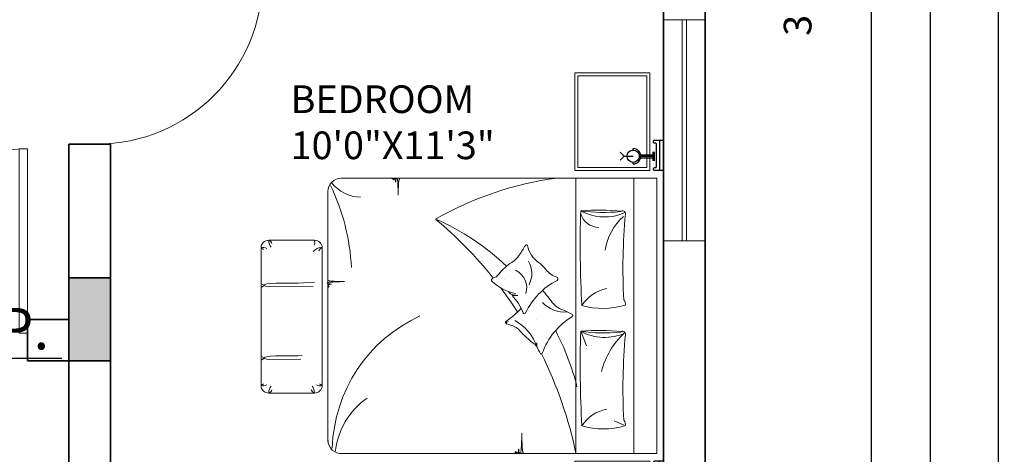
# Model space of a CAD drawing. Units: inches. Extents: x 3321 to 5237, y 11 to 1752.
# Tile 6 of 43: x 3652 to 3866, y 1204 to 1298. Entities that reach past the tile are written whole.
import ezdxf

# ---------------------------------------------------------------- set-up
doc = ezdxf.new("R2010")
doc.units = ezdxf.units.IN
for name, color, linetype, lineweight in [('A-ANNO-DIMS', 2, 'Continuous', 18), ('A-ANNO-TEXT', 7, 'Continuous', 18), ('A-AREA-IDEN', 7, 'Continuous', 18), ('A-COLS', 1, 'Continuous', 35), ('A-DOOR', 4, 'Continuous', 18), ('A-GLAZ', 5, 'Continuous', 18), ('A-WALL', 7, 'Continuous', 35), ('C-PROP', 7, 'Continuous', 30), ('FUR', 42, 'Continuous', 18)]:
    doc.layers.add(name, color=color, linetype=linetype, lineweight=lineweight)
for name, color, linetype in [('CEIL', 4, 'Continuous'), ('ELEC', 4, 'Continuous'), ('wood', 26, 'Continuous')]:
    doc.layers.add(name, color=color, linetype=linetype)
doc.styles.get("Standard").update_dxf_attribs({"font": 'arial.ttf'})
doc.dimstyles.new('ISO-25', dxfattribs={"dimtxt": 9, "dimasz": 2.5, "dimexe": 1.25, "dimexo": 0.625, "dimtad": 1, "dimdec": 1, "dimlunit": 3, "dimtxsty": 'Standard', "dimcen": 2.5, "dimclrd": 4, "dimclre": 4, "dimclrt": 256, "dimadec": 0, "dimazin": 0, "dimtfac": 1, "dimtdec": 1, "dimtmove": 0, "dimatfit": 3, "dimfxl": 1, "dimarcsym": 0})

# ---------------------------------------------------------------- blocks, each defined once
blk = doc.blocks.new('*U2')
for p, q in [((0, 0), (0, -6)), ((-40, 0), (-40, -6))]:
    blk.add_line(p, q)
blk.add_lwpolyline([(0, 0), (0, 40), (-1.75, 40), (-1.75, 0)], close=True)
blk.add_arc((0, 0), 40, 90, 180)
blk = doc.blocks.new('*U3')
for p, q in [((0, 0), (0, -6)), ((36, 0), (36, -6))]:
    blk.add_line(p, q)
blk.add_lwpolyline([(0, 0), (0, 36), (1.75, 36), (1.75, 0)], close=True)
blk.add_arc((0, 0), 36, 0, 90)
blk = doc.blocks.new('*D42')
at = {"layer": 'A-ANNO-DIMS', "color": 0, "lineweight": -2, "transparency": 16777216}
for p, q in [((3837.31, 1635.34), (3850.8, 1635.34)), ((3849.55, 1632.84), (3849.55, 1093.84)), ((3837.31, 1091.34), (3850.8, 1091.34))]:
    blk.add_line(p, q, dxfattribs=at)
at = {"layer": 'A-ANNO-DIMS', "color": 0, "transparency": 16777216}
for points in [[(3849.13, 1632.84), (3849.96, 1632.84), (3849.55, 1635.34)], [(3849.13, 1093.84), (3849.96, 1093.84), (3849.55, 1091.34)]]:
    blk.add_solid(points, dxfattribs=at)
at = {"layer": 'Defpoints', "color": 0, "transparency": 16777216}
for p in [(3836.69, 1635.34), (3836.69, 1091.34), (3849.55, 1091.34)]:
    blk.add_point(p, dxfattribs=at)
at = {"layer": 'A-ANNO-DIMS', "color": 0, "transparency": 16777216, "insert": (3844.35, 1363.34), "char_height": 9, "attachment_point": 5, "rotation": 90}
blk.add_mtext('45\'-4"', dxfattribs=at)
blk = doc.blocks.new('*D47')
at = {"layer": 'A-ANNO-DIMS', "color": 0, "lineweight": -2, "transparency": 16777216}
for p, q in [((3837.31, 1707.34), (3865.6, 1707.34)), ((3864.35, 989.84), (3864.35, 1704.84)), ((3837.31, 987.34), (3865.6, 987.34))]:
    blk.add_line(p, q, dxfattribs=at)
at = {"layer": 'A-ANNO-DIMS', "color": 0, "transparency": 16777216}
for points in [[(3863.93, 1704.84), (3864.76, 1704.84), (3864.35, 1707.34)], [(3863.93, 989.84), (3864.76, 989.84), (3864.35, 987.34)]]:
    blk.add_solid(points, dxfattribs=at)
at = {"layer": 'Defpoints', "color": 0, "transparency": 16777216}
for p in [(3836.69, 1707.34), (3864.35, 1707.34), (3836.69, 987.34)]:
    blk.add_point(p, dxfattribs=at)
at = {"layer": 'A-ANNO-DIMS', "color": 0, "transparency": 16777216, "insert": (3859.13, 1347.34), "char_height": 9, "attachment_point": 5, "rotation": 90}
blk.add_mtext("60'", dxfattribs=at)
blk = doc.blocks.new('*X127')
at = {"color": 0}
for p, q in [((3155.9, 8182.9), (3155.9, 8182.9)), ((3147.8, 8143.4), (3147.8, 8143.4)), ((3283, 8049.6), (3283, 8049.6)), ((3209.5, 8023.9), (3209.5, 8023.9)), ((3251.6, 7997), (3251.6, 7997)), ((3154.1, 7950.7), (3154.1, 7950.7))]:
    blk.add_line(p, q, dxfattribs=at)
blk = doc.blocks.new('*X126')
at = {"color": 0}
for p, q in [((3155.9, 8182.9), (3155.9, 8182.9)), ((3139.8, 7939.7), (3139.8, 7939.7))]:
    blk.add_line(p, q, dxfattribs=at)
blk = doc.blocks.new('*X125')
at = {"color": 0}
for p, q in [((3155.9, 8182.9), (3155.9, 8182.9)), ((3139.8, 7939.7), (3139.8, 7939.7))]:
    blk.add_line(p, q, dxfattribs=at)
blk = doc.blocks.new('*X124')
at = {"color": 0}
for p, q in [((3163, 7776.2), (3163, 7776.2)), ((3422.2, 7761.3), (3422.2, 7761.3)), ((3236.2, 7675.7), (3236.2, 7675.7)), ((3244.3, 7698.6), (3244.3, 7698.6)), ((3340.3, 7689.4), (3340.3, 7689.4))]:
    blk.add_line(p, q, dxfattribs=at)
blk = doc.blocks.new('BED1')
for p, q in [((0, -1000), (0, 800)), ((150, 800), (0, 800)), ((150, 800), (150, -1000)), ((2058.7, 800), (150, 800)), ((528, 800), (528, -1000)), ((211.8, 614.9), (277.5, 585.4)), ((2537.2, 404.9), (2237.2, 404.9)), ((2187.2, 354.9), (2187.2, -545.1)), ((2587.2, -545.1), (2587.2, 354.9)), ((2566.3, 178.5), (2565.2, 177.4)), ((2582, 188.1), (2565.4, 174.8)), ((2565.4, 174.8), (2585.7, 165.4)), ((2566.3, -296.8), (2565.2, -297.9)), ((2582, -287.1), (2565.4, -300.5)), ((2565.4, -300.5), (2585.7, -309.9)), ((2237.2, -595.1), (2537.2, -595.1)), ((150, -1000), (0, -1000)), ((150, -1000), (2063.5, -1000))]:
    blk.add_line(p, q)
for points in [[(934, 797.9), (930.9, 797.7), (928.3, 797.4), (926.3, 796.9), (924.9, 796.3), (923.8, 795.6), (923.1, 794.8), (922.7, 793.8), (922.5, 792.7), (922.4, 791.5), (922.5, 790.3), (922.6, 789.2), (922.6, 788.3), (922.6, 787.6), (922.4, 787.3), (922, 787.4), (921.4, 787.9), (920.6, 788.9), (919.5, 790.2), (918.4, 791.6), (917.1, 793.1), (915.9, 794.6), (914.6, 796), (913.3, 797.1), (912.2, 797.9), (911.1, 798.3), (910.1, 798.4), (909.2, 798), (908.3, 797.1), (907.5, 795.8), (906.8, 793.9), (906, 791.4), (905.4, 788.5), (904.8, 785.2), (904.2, 781.7), (903.7, 778.4), (903.2, 775.4), (902.8, 772.9), (902.5, 771.3), (902.3, 770.6), (902.1, 771.2), (902, 772.8), (901.8, 775.2), (901.7, 778.1), (901.5, 781.5), (901.2, 785), (900.8, 788.4), (900.2, 791.5), (899.5, 794.1), (898.6, 796.2), (897.6, 797.9), (896.5, 799.2), (895.3, 800), (894.1, 800.5), (893, 800.7), (891.9, 800.5), (890.9, 800.1), (890, 799), (889.1, 797.1), (888.3, 794), (887.6, 789.3), (886.9, 782.9), (886.2, 774.2), (885.5, 763.1), (884.8, 749.5), (884.2, 734.2), (883.6, 718.3), (883, 702.8), (882.5, 688.8), (882, 677.5), (881.7, 669.8), (881.5, 666.9), (881.3, 669.4), (881.3, 676.7), (881.3, 687.8), (881.2, 701.5), (881.1, 716.8), (880.8, 732.6), (880.2, 748), (879.4, 761.8), (878.3, 773.2), (876.9, 782.2), (875.1, 789.2), (872.9, 794.4), (870.3, 798), (869, 799)], [(2150, -913.5), (2150, 723.2)], [(2327.6, 182.3), (2530, 185.9), (2550.8, 181.9), (2561.7, 179), (2566, 176.7), (2566.9, 174.4), (2566.3, 171.9), (2562, 169.2), (2550.3, 166.5), (2527.7, 163.9), (2490.6, 161.8), (2345.5, 160.2), (2317.8, 158.5)], [(494.7, 3.1), (458.9, 95.3)], [(2149.7, -259.9), (2150, -268.4), (2150.1, -274.1), (2150.1, -278.1), (2150, -281.4), (2149.8, -284), (2149.5, -286.1), (2149.1, -287.8), (2148.7, -289), (2148.1, -289.9), (2147.4, -290.5), (2146.6, -290.8), (2145.6, -291), (2144.6, -291), (2143.6, -291), (2142.7, -290.9), (2141.9, -290.9), (2141.4, -290.9), (2141.1, -291), (2141.2, -291.4), (2141.7, -291.9), (2142.5, -292.6), (2143.5, -293.4), (2144.7, -294.4), (2146, -295.4), (2147.2, -296.5), (2148.4, -297.6), (2149.3, -298.6), (2150, -299.6), (2150.3, -300.5), (2150.4, -301.3), (2150, -302.1), (2149.3, -302.8), (2148.2, -303.5), (2146.6, -304.1), (2144.6, -304.7), (2142.1, -305.2), (2139.3, -305.7), (2136.5, -306.2), (2133.7, -306.6), (2131.2, -307), (2129.2, -307.3), (2127.8, -307.6), (2127.3, -307.8), (2127.7, -308), (2129, -308.1), (2131, -308.2), (2133.5, -308.3), (2136.3, -308.5), (2139.2, -308.7), (2142, -309), (2144.6, -309.5), (2146.8, -310.1), (2148.6, -310.9), (2150, -311.7), (2151, -312.7), (2151.7, -313.6), (2152.1, -314.6), (2152.3, -315.6), (2152.2, -316.5), (2151.8, -317.3), (2150.9, -318.1), (2149.3, -318.8), (2146.7, -319.4), (2142.8, -320), (2137.4, -320.6), (2130.2, -321.2), (2121, -321.8), (2109.7, -322.3), (2096.9, -322.9), (2083.6, -323.4), (2070.7, -323.9), (2059.1, -324.3), (2049.6, -324.7), (2043.2, -325), (2040.8, -325.2), (2042.9, -325.3), (2049, -325.3), (2058.2, -325.3), (2069.6, -325.4), (2082.3, -325.5), (2095.6, -325.8), (2108.4, -326.2), (2119.9, -326.8), (2129.4, -327.8), (2136.9, -329), (2142.7, -330.5), (2147, -332.3), (2150, -334.4), (2150.9, -335.6)], [(2246.5, -294.4), (2530, -289.4), (2550.8, -293.4), (2561.7, -296.3), (2566, -298.6), (2566.9, -300.8), (2566.3, -303.4), (2562, -306.1), (2550.3, -308.8), (2527.7, -311.3), (2490.6, -313.5), (2345.5, -315), (2238.6, -321.8)], [(1733.7, -998.3), (1731.1, -998.1), (1729, -997.8), (1727.4, -997.4), (1726.1, -997), (1725.2, -996.4), (1724.7, -995.7), (1724.3, -994.8), (1724.1, -993.9), (1724.1, -992.9), (1724.1, -991.9), (1724.2, -991), (1724.2, -990.2), (1724.2, -989.7), (1724.1, -989.4), (1723.8, -989.5), (1723.2, -990), (1722.5, -990.8), (1721.7, -991.8), (1720.7, -993), (1719.7, -994.3), (1718.6, -995.5), (1717.5, -996.6), (1716.5, -997.6), (1715.5, -998.3), (1714.6, -998.6), (1713.8, -998.6), (1713, -998.3), (1712.3, -997.6), (1711.7, -996.5), (1711, -994.9), (1710.4, -992.9), (1709.9, -990.4), (1709.4, -987.6), (1708.9, -984.8), (1708.5, -982), (1708.1, -979.5), (1707.8, -977.4), (1707.5, -976.1), (1707.3, -975.5), (1707.1, -976), (1707, -977.3), (1706.9, -979.3), (1706.8, -981.8), (1706.7, -984.6), (1706.4, -987.5), (1706.1, -990.3), (1705.6, -992.9), (1705, -995.1), (1704.2, -996.9), (1703.4, -998.3), (1702.4, -999.3), (1701.5, -1000), (1700.5, -1000.4), (1699.6, -1000.6), (1698.7, -1000.4), (1697.8, -1000.1), (1697, -999.2), (1696.3, -997.6), (1695.7, -995), (1695.1, -991.1), (1694.5, -985.7), (1693.9, -978.5), (1693.3, -969.3), (1692.8, -957.9), (1692.2, -945.2), (1691.7, -931.9), (1691.2, -919), (1690.8, -907.4), (1690.4, -897.9), (1690.1, -891.5), (1689.9, -889.1), (1689.8, -891.2), (1689.8, -897.3), (1689.8, -906.5), (1689.7, -917.9), (1689.6, -930.6), (1689.4, -943.8), (1688.9, -956.6), (1688.3, -968.1), (1687.3, -977.6), (1686.1, -985.2), (1684.6, -991), (1682.8, -995.3), (1680.7, -998.3), (1679.6, -999.2)]]:
    blk.add_lwpolyline(points)
for points in [[(205.5, 619.6, 0.267769), (215.1, 582.4, -0.037739), (204.3, 21.8, 0.684696), (236.7, 5.5, -0.060702), (497.2, 0.1, -0.046649), (225.9, 3.1, -1.318436)], [(489.2, 619.6, 0.144019), (207.6, 617.9, 0.248643)], [(497.2, 0.1, 0.021276), (489.2, 619.6, -0.206383), (326.6, 509.4, 0.237198)], [(211.8, 12.8, 0.143972), (361.6, 262.9, 1.292232)], [(886.4, -150, -0.069098), (985, -66.5, 0.658965), (982.1, -48.7, -0.049789), (927.4, -29, -0.103757), (896.6, -5.4, 0.055725), (800.9, 83.3, -0.11866), (782.7, 104.9, 0.016811), (761.6, 143.9, 0.70791), (748.3, 144, -0.16964), (551.9, -96.6, 0.664036), (554, -110.7, 0.023706), (627, -144.7, -0.134834), (683.2, -188, 0.012748), (746.3, -267.4)], [(969.1, -259.1, 0.263265), (936.3, -236.9, -0.026108), (909.2, -233.2, 0.027613), (945.1, -234.2, -0.089259), (872.7, -120, 0.662242), (857.6, -119.3, -0.162037), (651.8, -332.7, 0.676499), (654, -354.5, -0.160513), (722.9, -401.5, 0.07473), (773.5, -450.3, -0.187721), (845.5, -559.9, 0.70791), (858.8, -561.4, -0.010003), (898.6, -497.3, -0.113819), (947.3, -450.2, 0.099539), (1032.5, -372.4, -0.173425), (1070.9, -346.4, 0.589988), (1076.2, -326.1, 0.137312), (923.9, -245.9, 0.137312)], [(205.5, -168.2, 0.267769), (215.1, -205.4, -0.037739), (204.3, -766, 0.684696), (236.7, -782.3, -0.060702), (497.2, -787.7, -0.046649), (225.9, -784.7, -1.318436)], [(489.2, -168.2, 0.144019), (207.6, -169.9, 0.248643)], [(497.2, -787.7, 0.021276), (489.2, -168.2, -0.206383), (326.6, -278.4, 0.237198)], [(1446, -733.4, -0.095039), (652.8, -1001.7)]]:
    blk.add_lwpolyline(points, format="xyb")
for centre, radius, start, end in [((3208.8, 1363.3), 2739.4, 191.86791, 206.32469), ((1608.1, 842.5), 496.3, 305.19014, 354.02057), ((2062.7, 713.7), 86.5, 0, 93.53765), ((1138.6, 793.9), 983.2, 294.60777, 358.30329), ((2237.2, 354.9), 50, 90, 180), ((2321.1, 409.7), 84.5, 185.61958, 217.13957), ((2227.5, 373.5), 32.8, 17.83305, 72.80048), ((2546.9, 373.5), 32.8, 107.19952, 162.16695), ((2453.3, 409.7), 84.5, 322.86043, 354.38042), ((2537.2, 354.9), 50, 0, 90), ((2098.7, 754.7), 1625, 193.90497, 207.81692), ((2201.9, 323.3), 34.8, 50.8413, 114.9586), ((2212.2, 381.5), 36.5, 226.80948, 258.3841), ((2572.5, 323.3), 34.8, 65.0414, 129.1587), ((2562.2, 381.5), 36.5, 281.6159, 313.19052), ((751.8, 88.7), 34.9, 336.83517, 27.72181), ((684.2, 86), 100.3, 353.675, 10.88198), ((1074.1, 198.8), 306.1, 197.86019, 241.51221), ((341.4, -277.7), 318.5, 60.71255, 115.00895), ((983.7, -79.5), 20.8, 73.79673, 130.45661), ((978.5, -68.6), 14.3, 39.7097, 85.9506), ((602.5, -324), 198.6, 43.20348, 95.05559), ((3208.8, 1363.3), 2739.4, 212.93136, 216.95099), ((981.1, -281.8), 131.1, 164.0372, 243.45361), ((980, -379), 163.4, 152.61037, 209.36102), ((3208.8, 1363.3), 2739.4, 218.63292, 229.94485), ((2098.7, 754.7), 1625, 226.58872, 246.3156), ((3402.5, -342.9), 1408.5, 182.99169, 205.68187), ((-34.4, -471.2), 376.5, 312.01178, 350.96348), ((2178, -513.5), 33, 286.18268, 338.13858), ((2237.2, -545.1), 50, 180, 270), ((2188.1, -476.2), 73, 269.45125, 322.80265), ((2271.1, -580.9), 35.8, 148.90546, 197.55407), ((2546.9, -563.8), 32.8, 197.83305, 252.80048), ((2453.3, -600), 84.5, 5.61958, 37.13957), ((2537.2, -545.1), 50, 270, 0), ((2572.5, -513.6), 34.8, 230.8413, 294.9586), ((2562.2, -571.8), 36.5, 46.80948, 78.3841), ((375.7, -807.4), 128.2, 17.40732, 88.51286), ((341.4, -1065.5), 318.5, 60.71255, 115.00895), ((1929.1, -1126), 250.5, 37.85533, 88.44053), ((2063.5, -913.5), 86.5, 270, 0)]:
    blk.add_arc(centre, radius, start, end)
for name in ['*X126', '*X125', '*X127', '*X124']:
    blk.add_blockref(name, (-2425.3, -8101.4))
blk = doc.blocks.new('APLIQ')
at = {"layer": 'ELEC'}
for p, q in [((0, 0.2), (-0.0261, 0.2261)), ((0, 0.2), (0.0261, 0.2261)), ((0, 0.2), (0, 0.14)), ((-0.05, 0.14), (-0.04, 0.14)), ((0.04, 0.14), (0.05, 0.14)), ((-0.01, 0.09), (-0.01, 0.01)), ((0, 0.09), (0, 0)), ((0.01, 0.09), (0.01, 0.01)), ((-0.03, 0.01), (0.03, 0.01)), ((-0.03, 0), (0.03, 0))]:
    blk.add_line(p, q, dxfattribs=at)
blk.add_circle((0, 0.14), 0.04, dxfattribs=at)
blk.add_arc((0, 0.14), 0.05, 180, 0, dxfattribs=at)
blk = doc.blocks.new('A$C68AE1801')
at = {"layer": 'FUR'}
for points in [[(2.5416, 3.18), (2.5416, 2.54), (2.0516, 2.54), (2.0516, 3.18)], [(2.5216, 3.16), (2.5216, 2.56), (2.0716, 2.56), (2.0716, 3.16)], [(2.5416, 0), (2.5416, 0.64), (2.0516, 0.64), (2.0516, 0)], [(2.5216, 0.02), (2.5216, 0.62), (2.0716, 0.62), (2.0716, 0.02)]]:
    blk.add_lwpolyline(points, close=True, dxfattribs=at)
at = {"layer": 'wood'}
for p, q in [((2.6057, 2.74), (2.6057, 2.54)), ((2.6057, 0.44), (2.6057, 0.64))]:
    blk.add_line(p, q, dxfattribs=at)
for points in [[(2.5657, 2.728), (2.5657, 2.732, -0.414214), (2.5737, 2.74), (2.6321, 2.74), (2.6321, 2.54), (2.5737, 2.54, -0.414214), (2.5657, 2.548), (2.5657, 2.552, -0.414214), (2.5737, 2.56), (2.5777, 2.56, 0.414214), (2.5857, 2.568), (2.5857, 2.712, 0.414214), (2.5777, 2.72), (2.5737, 2.72, -0.414214)], [(2.5657, 0.452), (2.5657, 0.448, 0.414214), (2.5737, 0.44), (2.6321, 0.44), (2.6321, 0.64), (2.5737, 0.64, 0.414214), (2.5657, 0.632), (2.5657, 0.628, 0.414214), (2.5737, 0.62), (2.5777, 0.62, -0.414214), (2.5857, 0.612), (2.5857, 0.468, -0.414214), (2.5777, 0.46), (2.5737, 0.46, 0.414214)]]:
    blk.add_lwpolyline(points, format="xyb", close=True, dxfattribs=at)
at = {"layer": 'CEIL', "rotation": 90}
blk.add_blockref('APLIQ', (2.5736, 2.634), dxfattribs=at)
at = {"layer": 'CEIL', "xscale": -1, "rotation": 90}
blk.add_blockref('APLIQ', (2.5736, 0.546), dxfattribs=at)
at = {"layer": 'FUR', "xscale": 0.001, "yscale": 0.001, "zscale": 0.001, "rotation": 180}
blk.add_blockref('BED1', (2.5872, 1.49), dxfattribs=at)
blk = doc.blocks.new('COL-9X18-IN')
h = blk.add_hatch(color=256)
h.dxf.hatch_style = 1
h.paths.add_polyline_path([(9, 18), (0, 18), (0, 0), (9, 0)])
blk.add_lwpolyline([(0, 0), (9, 0), (9, 18), (0, 18)], close=True)
blk = doc.blocks.new('WIN-48IN-9IN-WALL')
for p, q in [((0, 0), (0, 9)), ((48, 0), (48, 9)), ((0, 5), (48, 5)), ((0, 4), (48, 4))]:
    blk.add_line(p, q)
blk = doc.blocks.new('PROPERTY-40X60FT')
blk.add_line((480, 720), (480, 0))
blk = doc.blocks.new('*D207')
at = {"layer": 'A-ANNO-DIMS', "color": 4, "lineweight": -2, "transparency": 16777216}
for p, q in [((3510, 1232.49), (3510, 1223.64)), ((3564.86, 1232.49), (3564.86, 1223.64)), ((3512.5, 1224.89), (3562.36, 1224.89)), ((3564.86, 1224.89), (3661.15, 1224.89))]:
    blk.add_line(p, q, dxfattribs=at)
at = {"layer": 'A-ANNO-DIMS', "color": 4, "transparency": 16777216}
for points in [[(3512.5, 1225.31), (3512.5, 1224.47), (3510, 1224.89)], [(3562.36, 1225.31), (3562.36, 1224.47), (3564.86, 1224.89)]]:
    blk.add_solid(points, dxfattribs=at)
at = {"layer": 'Defpoints', "color": 0, "transparency": 16777216}
for p in [(3510, 1233.12), (3564.86, 1233.12), (3564.86, 1224.89)]:
    blk.add_point(p, dxfattribs=at)
at = {"layer": 'A-ANNO-DIMS', "transparency": 16777216, "insert": (3614.25, 1230.17), "char_height": 9, "attachment_point": 5}
blk.add_mtext('SOFA 4\'-7" TYP.', dxfattribs=at)

msp = doc.modelspace()

# ---------------------------------------------------------------- linework, layer by layer
at = {"layer": 'A-WALL'}
for p, q in [((3800.69, 1635.34), (3800.69, 1091.34)), ((3791.69, 1316.34), (3791.69, 1181.34)), ((3662.69, 1271.34), (3671.69, 1271.34)), ((3662.69, 1271.34), (3662.69, 1233.34)), ((3671.69, 1271.34), (3671.69, 1181.34)), ((3653.69, 1233.34), (3653.69, 1224.34)), ((3653.69, 1233.34), (3662.69, 1233.34)), ((3653.69, 1224.34), (3662.69, 1224.34)), ((3662.69, 1224.34), (3662.69, 1172.34))]:
    msp.add_line(p, q, dxfattribs=at)

# ---------------------------------------------------------------- block references
at = {"layer": 'A-COLS', "rotation": 180}
msp.add_blockref('COL-9X18-IN', (3671.69, 1242.34), dxfattribs=at)
at = {"layer": 'A-DOOR', "rotation": 270}
msp.add_blockref('*U3', (3668.69, 1307.34), dxfattribs=at)
at = {"layer": 'A-DOOR'}
msp.add_blockref('*U2', (3653.69, 1230.34), dxfattribs=at)
at = {"layer": 'A-GLAZ', "rotation": 89.9999999999993}
msp.add_blockref('WIN-48IN-9IN-WALL', (3800.69, 1250.34), dxfattribs=at)
at = {"layer": 'C-PROP'}
msp.add_blockref('PROPERTY-40X60FT', (3356.69, 987.34), dxfattribs=at)
at = {"layer": 'FUR', "xscale": 33.17188472218209, "yscale": 33.17188472218209, "zscale": 33.17188472218209}
msp.add_blockref('A$C68AE1801', (3704.38, 1181.34), dxfattribs=at)

# ---------------------------------------------------------------- texts
at = {"layer": 'A-ANNO-TEXT', "insert": (3817.76, 1294.84), "char_height": 6, "attachment_point": 1, "rotation": 90}
msp.add_mtext_dynamic_manual_height_columns('3\'0" SETBACK', width=97.3114, gutter_width=25, heights=[0], dxfattribs=at)
at = {"layer": 'A-AREA-IDEN', "insert": (3710.8, 1284.09), "char_height": 6, "attachment_point": 1}
msp.add_mtext_dynamic_manual_height_columns('BEDROOM\\P10\'0"X11\'3"', width=97.3114, gutter_width=25, heights=[0], dxfattribs=at)

# ---------------------------------------------------------------- dimensions: what is measured, and where the dimension line sits
at = {"layer": 'A-ANNO-DIMS'}
for base, p1, p2, angle, override, picture, middle in [((3864.35, 1707.34), (3836.69, 987.34), (3836.69, 1707.34), 270, {"dimclrd": 0, "dimclre": 0, "dimclrt": 0}, '*D47', (3859.13, 1347.34)), ((3849.55, 1091.34), (3836.69, 1635.34), (3836.69, 1091.34), 90, {"dimclrd": 0, "dimclre": 0, "dimclrt": 0, "dimtmove": 1}, '*D42', (3844.35, 1363.34))]:
    dim = msp.add_linear_dim(base=base, p1=p1, p2=p2, angle=angle, dimstyle='ISO-25', override=override, dxfattribs=at)
    dim.commit()
    dim.dimension.update_dxf_attribs({"geometry": picture, "text_midpoint": middle})
dim = msp.add_linear_dim(base=(3564.86, 1224.89), p1=(3510, 1233.12), p2=(3564.86, 1233.12), text='SOFA <> TYP.', dimstyle='ISO-25', override={"dimdec": 1, "dimlfac": 1, "dimrnd": 0, "dimzin": 1, "dimdsep": 46, "dimlunit": 4, "dimfrac": 2}, dxfattribs=at)
dim.commit()
dim.dimension.update_dxf_attribs({"geometry": '*D207', "text_midpoint": (3614.25, 1230.17)})

doc.saveas('drawing.dxf')
